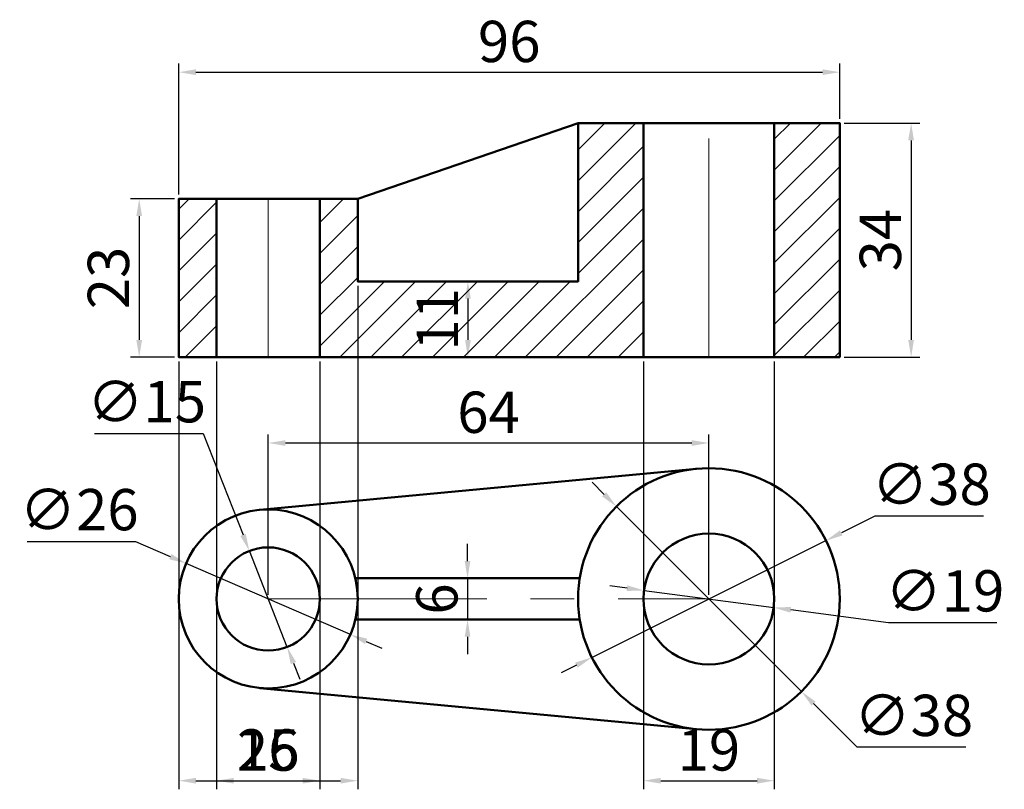
# Model space of a CAD drawing. Units: millimetres. Extents: x 5 to 148, y 12 to 123.
import ezdxf

# ---------------------------------------------------------------- set-up
doc = ezdxf.new("R2010")
doc.units = ezdxf.units.MM
doc.linetypes.add('CENTER', pattern=[50.8, 31.75, -6.35, 6.35, -6.35])
for name, color, linetype, lineweight in [('M-CNTR', 4, 'CENTER', 18), ('M-DIMS', 2, 'Continuous', 25), ('M-HATC', 8, 'Continuous', 18), ('M-OUTL', 7, 'Continuous', 50)]:
    doc.layers.add(name, color=color, linetype=linetype, lineweight=lineweight)
doc.styles.get("Standard").update_dxf_attribs({"font": 'arial.ttf'})
doc.dimstyles.new('ISO-25', dxfattribs={"dimtxt": 6, "dimasz": 2.5, "dimexe": 1.25, "dimexo": 0.625, "dimtad": 1, "dimtoh": 1, "dimdec": 0, "dimtxsty": 'Standard', "dimcen": 2.5, "dimadec": 0, "dimazin": 0, "dimtfac": 1, "dimtdec": 0, "dimtmove": 0, "dimatfit": 3, "dimfxl": 1, "dimarcsym": 0})

# ---------------------------------------------------------------- blocks, each defined once
blk = doc.blocks.new('*D1')
at = {"layer": 'Defpoints', "color": 0, "transparency": 16777216}
for p in [(28.54, 97.39), (22.8, 74.39), (28.54, 74.39)]:
    blk.add_point(p, dxfattribs=at)
at = {"layer": 'M-DIMS', "color": 0, "lineweight": -2, "transparency": 16777216}
for p, q in [((27.92, 97.39), (21.55, 97.39)), ((22.8, 94.89), (22.8, 76.89)), ((27.92, 74.39), (21.55, 74.39))]:
    blk.add_line(p, q, dxfattribs=at)
at = {"layer": 'M-DIMS', "color": 0, "transparency": 16777216}
for points in [[(22.39, 94.89), (23.22, 94.89), (22.8, 97.39)], [(22.39, 76.89), (23.22, 76.89), (22.8, 74.39)]]:
    blk.add_solid(points, dxfattribs=at)
at = {"layer": 'M-DIMS', "color": 0, "transparency": 16777216, "insert": (19.11, 85.89), "char_height": 6, "attachment_point": 5, "rotation": 90}
blk.add_mtext('23', dxfattribs=at)
blk = doc.blocks.new('*D2')
at = {"layer": 'Defpoints', "color": 0, "transparency": 16777216}
for p in [(124.54, 108.39), (124.54, 74.39), (134.91, 74.39)]:
    blk.add_point(p, dxfattribs=at)
at = {"layer": 'M-DIMS', "color": 0, "lineweight": -2, "transparency": 16777216}
for p, q in [((125.17, 108.39), (136.16, 108.39)), ((134.91, 105.89), (134.91, 76.89)), ((125.17, 74.39), (136.16, 74.39))]:
    blk.add_line(p, q, dxfattribs=at)
at = {"layer": 'M-DIMS', "color": 0, "transparency": 16777216}
for points in [[(134.49, 105.89), (135.32, 105.89), (134.91, 108.39)], [(134.49, 76.89), (135.32, 76.89), (134.91, 74.39)]]:
    blk.add_solid(points, dxfattribs=at)
at = {"layer": 'M-DIMS', "color": 0, "transparency": 16777216, "insert": (131.22, 91.39), "char_height": 6, "attachment_point": 5, "rotation": 90}
blk.add_mtext('34', dxfattribs=at)
blk = doc.blocks.new('*D3')
at = {"layer": 'Defpoints', "color": 0, "transparency": 16777216}
for p in [(70.54, 85.39), (70.54, 74.39), (70.54, 74.39)]:
    blk.add_point(p, dxfattribs=at)
at = {"layer": 'M-DIMS', "color": 0, "lineweight": -2, "transparency": 16777216}
for p, q in [((71.17, 85.39), (71.79, 85.39)), ((70.54, 82.89), (70.54, 76.89)), ((71.17, 74.39), (71.79, 74.39))]:
    blk.add_line(p, q, dxfattribs=at)
at = {"layer": 'M-DIMS', "color": 0, "transparency": 16777216}
for points in [[(70.13, 82.89), (70.96, 82.89), (70.54, 85.39)], [(70.13, 76.89), (70.96, 76.89), (70.54, 74.39)]]:
    blk.add_solid(points, dxfattribs=at)
at = {"layer": 'M-DIMS', "color": 0, "transparency": 16777216, "insert": (66.9, 79.89), "char_height": 6, "attachment_point": 5, "rotation": 90}
blk.add_mtext('11', dxfattribs=at)
blk = doc.blocks.new('*D4')
at = {"layer": 'Defpoints', "color": 0, "transparency": 16777216}
for p in [(105.54, 61.92), (41.54, 39.26), (105.54, 39.26)]:
    blk.add_point(p, dxfattribs=at)
at = {"layer": 'M-DIMS', "color": 0, "lineweight": -2, "transparency": 16777216}
for p, q in [((41.54, 39.88), (41.54, 63.17)), ((105.54, 39.88), (105.54, 63.17)), ((44.04, 61.92), (103.04, 61.92))]:
    blk.add_line(p, q, dxfattribs=at)
at = {"layer": 'M-DIMS', "color": 0, "transparency": 16777216}
for points in [[(44.04, 62.33), (44.04, 61.5), (41.54, 61.92)], [(103.04, 62.33), (103.04, 61.5), (105.54, 61.92)]]:
    blk.add_solid(points, dxfattribs=at)
at = {"layer": 'M-DIMS', "color": 0, "transparency": 16777216, "insert": (73.54, 65.61), "char_height": 6, "attachment_point": 5}
blk.add_mtext('64', dxfattribs=at)
blk = doc.blocks.new('*D5')
at = {"layer": 'Defpoints', "color": 0, "transparency": 16777216}
for p in [(70.49, 42.26), (70.49, 36.26), (70.49, 36.26)]:
    blk.add_point(p, dxfattribs=at)
at = {"layer": 'M-DIMS', "color": 0, "lineweight": -2, "transparency": 16777216}
for p, q in [((70.49, 44.76), (70.49, 47.26)), ((69.86, 42.26), (69.24, 42.26)), ((70.49, 42.26), (70.49, 36.26)), ((69.86, 36.26), (69.24, 36.26)), ((70.49, 33.76), (70.49, 31.26))]:
    blk.add_line(p, q, dxfattribs=at)
at = {"layer": 'M-DIMS', "color": 0, "transparency": 16777216}
for points in [[(70.07, 44.76), (70.9, 44.76), (70.49, 42.26)], [(70.07, 33.76), (70.9, 33.76), (70.49, 36.26)]]:
    blk.add_solid(points, dxfattribs=at)
at = {"layer": 'M-DIMS', "color": 0, "transparency": 16777216, "insert": (66.8, 39.26), "char_height": 6, "attachment_point": 5, "rotation": 90}
blk.add_mtext('6', dxfattribs=at)
blk = doc.blocks.new('*D6')
at = {"layer": 'Defpoints', "color": 0, "transparency": 16777216}
for p in [(29.61, 44.42), (53.47, 34.09)]:
    blk.add_point(p, dxfattribs=at)
at = {"layer": 'M-DIMS', "color": 0, "lineweight": -2, "transparency": 16777216}
for p, q in [((6.52, 47.6), (22.27, 47.6)), ((22.27, 47.6), (27.32, 45.41)), ((53.47, 34.09), (29.61, 44.42)), ((55.77, 33.1), (58.06, 32.11))]:
    blk.add_line(p, q, dxfattribs=at)
at = {"layer": 'M-DIMS', "color": 0, "transparency": 16777216}
for points in [[(27.48, 45.8), (27.15, 45.03), (29.61, 44.42)], [(55.93, 33.48), (55.6, 32.72), (53.47, 34.09)]]:
    blk.add_solid(points, dxfattribs=at)
at = {"layer": 'M-DIMS', "color": 0, "transparency": 16777216, "insert": (14.08, 51.46), "char_height": 6, "attachment_point": 5}
blk.add_mtext('∅26', dxfattribs=at)
blk = doc.blocks.new('*D7')
at = {"layer": 'Defpoints', "color": 0, "transparency": 16777216}
for p in [(38.8, 46.24), (44.29, 32.28)]:
    blk.add_point(p, dxfattribs=at)
at = {"layer": 'M-DIMS', "color": 0, "lineweight": -2, "transparency": 16777216}
for p, q in [((16.3, 63.28), (32.09, 63.28)), ((32.09, 63.28), (37.88, 48.56)), ((44.29, 32.28), (38.8, 46.24)), ((45.2, 29.95), (46.12, 27.62))]:
    blk.add_line(p, q, dxfattribs=at)
at = {"layer": 'M-DIMS', "color": 0, "transparency": 16777216}
for points in [[(38.27, 48.72), (37.49, 48.41), (38.8, 46.24)], [(45.59, 30.1), (44.81, 29.8), (44.29, 32.28)]]:
    blk.add_solid(points, dxfattribs=at)
at = {"layer": 'M-DIMS', "color": 0, "transparency": 16777216, "insert": (23.88, 67.14), "char_height": 6, "attachment_point": 5}
blk.add_mtext('∅15', dxfattribs=at)
blk = doc.blocks.new('*D8')
at = {"layer": 'Defpoints', "color": 0, "transparency": 16777216}
for p in [(122.54, 47.74), (88.54, 30.77)]:
    blk.add_point(p, dxfattribs=at)
at = {"layer": 'M-DIMS', "color": 0, "lineweight": -2, "transparency": 16777216}
for p, q in [((129.65, 51.29), (124.78, 48.86)), ((145.41, 51.29), (129.65, 51.29)), ((88.54, 30.77), (122.54, 47.74)), ((86.31, 29.65), (84.07, 28.53))]:
    blk.add_line(p, q, dxfattribs=at)
at = {"layer": 'M-DIMS', "color": 0, "transparency": 16777216}
for points in [[(124.59, 49.23), (124.96, 48.49), (122.54, 47.74)], [(86.12, 30.02), (86.49, 29.28), (88.54, 30.77)]]:
    blk.add_solid(points, dxfattribs=at)
at = {"layer": 'M-DIMS', "color": 0, "transparency": 16777216, "insert": (137.84, 55.15), "char_height": 6, "attachment_point": 5}
blk.add_mtext('∅38', dxfattribs=at)
blk = doc.blocks.new('*D9')
at = {"layer": 'Defpoints', "color": 0, "transparency": 16777216}
for p in [(96.12, 40.5), (114.96, 38.01)]:
    blk.add_point(p, dxfattribs=at)
at = {"layer": 'M-DIMS', "color": 0, "lineweight": -2, "transparency": 16777216}
for p, q in [((93.65, 40.83), (91.17, 41.16)), ((96.12, 40.5), (114.96, 38.01)), ((131.61, 35.81), (117.44, 37.68)), ((147.37, 35.81), (131.61, 35.81))]:
    blk.add_line(p, q, dxfattribs=at)
at = {"layer": 'M-DIMS', "color": 0, "transparency": 16777216}
for points in [[(93.7, 41.24), (93.59, 40.42), (96.12, 40.5)], [(117.49, 38.1), (117.38, 37.27), (114.96, 38.01)]]:
    blk.add_solid(points, dxfattribs=at)
at = {"layer": 'M-DIMS', "color": 0, "transparency": 16777216, "insert": (139.81, 39.66), "char_height": 6, "attachment_point": 5}
blk.add_mtext('∅19', dxfattribs=at)
blk = doc.blocks.new('*D10')
at = {"layer": 'Defpoints', "color": 0, "transparency": 16777216}
for p in [(54.54, 85.39), (28.54, 74.39), (54.54, 12.86)]:
    blk.add_point(p, dxfattribs=at)
at = {"layer": 'M-DIMS', "color": 0, "lineweight": -2, "transparency": 16777216}
for p, q in [((54.54, 84.77), (54.54, 11.61)), ((28.54, 73.77), (28.54, 11.61)), ((31.04, 12.86), (52.04, 12.86))]:
    blk.add_line(p, q, dxfattribs=at)
at = {"layer": 'M-DIMS', "color": 0, "transparency": 16777216}
for points in [[(31.04, 13.27), (31.04, 12.44), (28.54, 12.86)], [(52.04, 13.27), (52.04, 12.44), (54.54, 12.86)]]:
    blk.add_solid(points, dxfattribs=at)
at = {"layer": 'M-DIMS', "color": 0, "transparency": 16777216, "insert": (41.54, 16.55), "char_height": 6, "attachment_point": 5}
blk.add_mtext('26', dxfattribs=at)
blk = doc.blocks.new('*D11')
at = {"layer": 'Defpoints', "color": 0, "transparency": 16777216}
for p in [(34.04, 74.39), (49.04, 74.39), (49.04, 12.86)]:
    blk.add_point(p, dxfattribs=at)
at = {"layer": 'M-DIMS', "color": 0, "lineweight": -2, "transparency": 16777216}
for p, q in [((34.04, 73.77), (34.04, 11.61)), ((49.04, 73.77), (49.04, 11.61)), ((36.54, 12.86), (46.54, 12.86))]:
    blk.add_line(p, q, dxfattribs=at)
at = {"layer": 'M-DIMS', "color": 0, "transparency": 16777216}
for points in [[(36.54, 13.27), (36.54, 12.44), (34.04, 12.86)], [(46.54, 13.27), (46.54, 12.44), (49.04, 12.86)]]:
    blk.add_solid(points, dxfattribs=at)
at = {"layer": 'M-DIMS', "color": 0, "transparency": 16777216, "insert": (41.54, 16.55), "char_height": 6, "attachment_point": 5}
blk.add_mtext('15', dxfattribs=at)
blk = doc.blocks.new('*D12')
at = {"layer": 'Defpoints', "color": 0, "transparency": 16777216}
for p in [(96.04, 74.39), (115.04, 74.39), (115.04, 12.86)]:
    blk.add_point(p, dxfattribs=at)
at = {"layer": 'M-DIMS', "color": 0, "lineweight": -2, "transparency": 16777216}
for p, q in [((96.04, 73.77), (96.04, 11.61)), ((115.04, 73.77), (115.04, 11.61)), ((98.54, 12.86), (112.54, 12.86))]:
    blk.add_line(p, q, dxfattribs=at)
at = {"layer": 'M-DIMS', "color": 0, "transparency": 16777216}
for points in [[(98.54, 13.27), (98.54, 12.44), (96.04, 12.86)], [(112.54, 13.27), (112.54, 12.44), (115.04, 12.86)]]:
    blk.add_solid(points, dxfattribs=at)
at = {"layer": 'M-DIMS', "color": 0, "transparency": 16777216, "insert": (105.54, 16.55), "char_height": 6, "attachment_point": 5}
blk.add_mtext('19', dxfattribs=at)
blk = doc.blocks.new('*D13')
at = {"layer": 'Defpoints', "color": 0, "transparency": 16777216}
for p in [(124.54, 115.79), (124.54, 108.39), (28.54, 97.39)]:
    blk.add_point(p, dxfattribs=at)
at = {"layer": 'M-DIMS', "color": 0, "lineweight": -2, "transparency": 16777216}
for p, q in [((28.54, 98.02), (28.54, 117.04)), ((124.54, 109.02), (124.54, 117.04)), ((31.04, 115.79), (122.04, 115.79))]:
    blk.add_line(p, q, dxfattribs=at)
at = {"layer": 'M-DIMS', "color": 0, "transparency": 16777216}
for points in [[(31.04, 116.21), (31.04, 115.38), (28.54, 115.79)], [(122.04, 116.21), (122.04, 115.38), (124.54, 115.79)]]:
    blk.add_solid(points, dxfattribs=at)
at = {"layer": 'M-DIMS', "color": 0, "transparency": 16777216, "insert": (76.54, 119.48), "char_height": 6, "attachment_point": 5}
blk.add_mtext('96', dxfattribs=at)
blk = doc.blocks.new('*D14')
at = {"layer": 'Defpoints', "color": 0, "transparency": 16777216}
for p in [(92.11, 52.69), (118.98, 25.82)]:
    blk.add_point(p, dxfattribs=at)
at = {"layer": 'M-DIMS', "color": 0, "lineweight": -2, "transparency": 16777216}
for p, q in [((90.34, 54.46), (88.57, 56.23)), ((92.11, 52.69), (118.98, 25.82)), ((127.08, 17.72), (120.75, 24.05)), ((142.84, 17.72), (127.08, 17.72))]:
    blk.add_line(p, q, dxfattribs=at)
at = {"layer": 'M-DIMS', "color": 0, "transparency": 16777216}
for points in [[(90.63, 54.75), (90.04, 54.16), (92.11, 52.69)], [(121.04, 24.35), (120.45, 23.76), (118.98, 25.82)]]:
    blk.add_solid(points, dxfattribs=at)
at = {"layer": 'M-DIMS', "color": 0, "transparency": 16777216, "insert": (135.28, 21.57), "char_height": 6, "attachment_point": 5}
blk.add_mtext('∅38', dxfattribs=at)

msp = doc.modelspace()

# ---------------------------------------------------------------- hatches: boundary and pattern name
at = {"layer": 'M-HATC'}
h = msp.add_hatch(dxfattribs=at)
h.set_pattern_fill('ANSI31', color=256)
h.paths.add_polyline_path([(34.04, 97.39), (28.54, 97.39), (28.54, 74.39), (34.04, 74.39)])
h.paths.add_polyline_path([(96.04, 108.39), (86.54, 108.39), (86.54, 85.39), (54.54, 85.39), (54.54, 97.39), (49.04, 97.39), (49.04, 74.39), (96.04, 74.39)])
h.paths.add_polyline_path([(124.54, 108.39), (115.04, 108.39), (115.04, 74.39), (124.54, 74.39)])

# ---------------------------------------------------------------- linework, layer by layer
at = {"layer": 'M-CNTR'}
for p, q in [((105.54, 74.39), (105.54, 108.39)), ((41.54, 74.39), (41.54, 97.39)), ((41.54, 39.26), (105.54, 39.26))]:
    msp.add_line(p, q, dxfattribs=at)
at = {"layer": 'M-OUTL'}
for p, q in [((96.04, 74.39), (96.04, 108.39)), ((115.04, 74.39), (115.04, 108.39)), ((34.04, 74.39), (34.04, 97.39)), ((49.04, 74.39), (49.04, 97.39)), ((40.32, 52.2), (103.76, 58.17)), ((54.19, 42.26), (86.78, 42.26)), ((54.19, 36.26), (86.78, 36.26)), ((40.32, 26.31), (103.76, 20.34))]:
    msp.add_line(p, q, dxfattribs=at)
msp.add_lwpolyline([(54.54, 97.39), (28.54, 97.39), (28.54, 74.39), (124.54, 74.39), (124.54, 108.39), (86.54, 108.39)], dxfattribs=at)
msp.add_lwpolyline([(54.54, 97.39), (86.54, 108.39), (86.54, 85.39), (54.54, 85.39)], close=True, dxfattribs=at)
for centre, radius in [((105.54, 39.26), 19), ((41.54, 39.26), 13), ((105.54, 39.26), 9.5), ((41.54, 39.26), 7.5)]:
    msp.add_circle(centre, radius, dxfattribs=at)

# ---------------------------------------------------------------- dimensions: what is measured, and where the dimension line sits
at = {"layer": 'M-DIMS'}
for base, p1, p2, override, picture, middle in [((124.54, 115.79), (28.54, 97.39), (124.54, 108.39), {"dimdec": 0, "dimlfac": 1, "dimrnd": 0, "dimzin": 0, "dimdsep": 46, "dimlunit": 2}, '*D13', (76.54, 119.48)), ((54.54, 12.86), (28.54, 74.39), (54.54, 85.39), {"dimdec": 0, "dimlfac": 1, "dimrnd": 0, "dimzin": 0, "dimdsep": 46, "dimlunit": 2}, '*D10', (41.54, 16.55)), ((49.04, 12.86), (34.04, 74.39), (49.04, 74.39), {"dimdec": 0, "dimlfac": 1, "dimrnd": 0, "dimzin": 0, "dimdsep": 46, "dimlunit": 2}, '*D11', (41.54, 16.55)), ((115.04, 12.86), (96.04, 74.39), (115.04, 74.39), {"dimdec": 0, "dimlfac": 1, "dimrnd": 0, "dimzin": 0, "dimdsep": 46, "dimlunit": 2}, '*D12', (105.54, 16.55)), ((105.54, 61.92), (41.54, 39.26), (105.54, 39.26), {"dimclrd": 0, "dimclre": 0, "dimclrt": 0}, '*D4', (73.54, 65.61))]:
    dim = msp.add_linear_dim(base=base, p1=p1, p2=p2, dimstyle='ISO-25', override=override, dxfattribs=at)
    dim.commit()
    dim.dimension.update_dxf_attribs({"geometry": picture, "text_midpoint": middle})
for base, p1, p2, picture, middle in [((134.91, 74.39), (124.54, 108.39), (124.54, 74.39), '*D2', (131.22, 91.39)), ((22.8, 74.39), (28.54, 97.39), (28.54, 74.39), '*D1', (19.11, 85.89)), ((70.54, 74.39), (70.54, 85.39), (70.54, 74.39), '*D3', (66.9, 79.89)), ((70.49, 36.26), (70.49, 42.26), (70.49, 36.26), '*D5', (66.8, 39.26))]:
    dim = msp.add_linear_dim(base=base, p1=p1, p2=p2, angle=90, dimstyle='ISO-25', override={"dimclrd": 0, "dimclre": 0, "dimclrt": 0}, dxfattribs=at)
    dim.commit()
    dim.dimension.update_dxf_attribs({"geometry": picture, "text_midpoint": middle})
for p1, p2, override, picture, middle in [((44.29, 32.28), (38.8, 46.24), {"dimclrd": 0, "dimclre": 0, "dimclrt": 0}, '*D7', (23.88, 63.28)), ((88.54, 30.77), (122.54, 47.74), {"dimclrd": 0, "dimclre": 0, "dimclrt": 0}, '*D8', (137.84, 51.29)), ((92.11, 52.69), (118.98, 25.82), {"dimdec": 0, "dimlfac": 1, "dimrnd": 0, "dimzin": 0, "dimdsep": 46, "dimlunit": 2}, '*D14', (135.28, 17.72)), ((53.47, 34.09), (29.61, 44.42), {"dimclrd": 0, "dimclre": 0, "dimclrt": 0}, '*D6', (14.08, 47.6)), ((96.12, 40.5), (114.96, 38.01), {"dimclrd": 0, "dimclre": 0, "dimclrt": 0}, '*D9', (131.61, 35.81))]:
    dim = msp.add_diameter_dim_2p(p1=p1, p2=p2, dimstyle='ISO-25', override=override, dxfattribs=at)
    dim.commit()
    dim.dimension.update_dxf_attribs({"geometry": picture, "text_midpoint": middle, "dimtype": 163})

doc.saveas('drawing.dxf')
